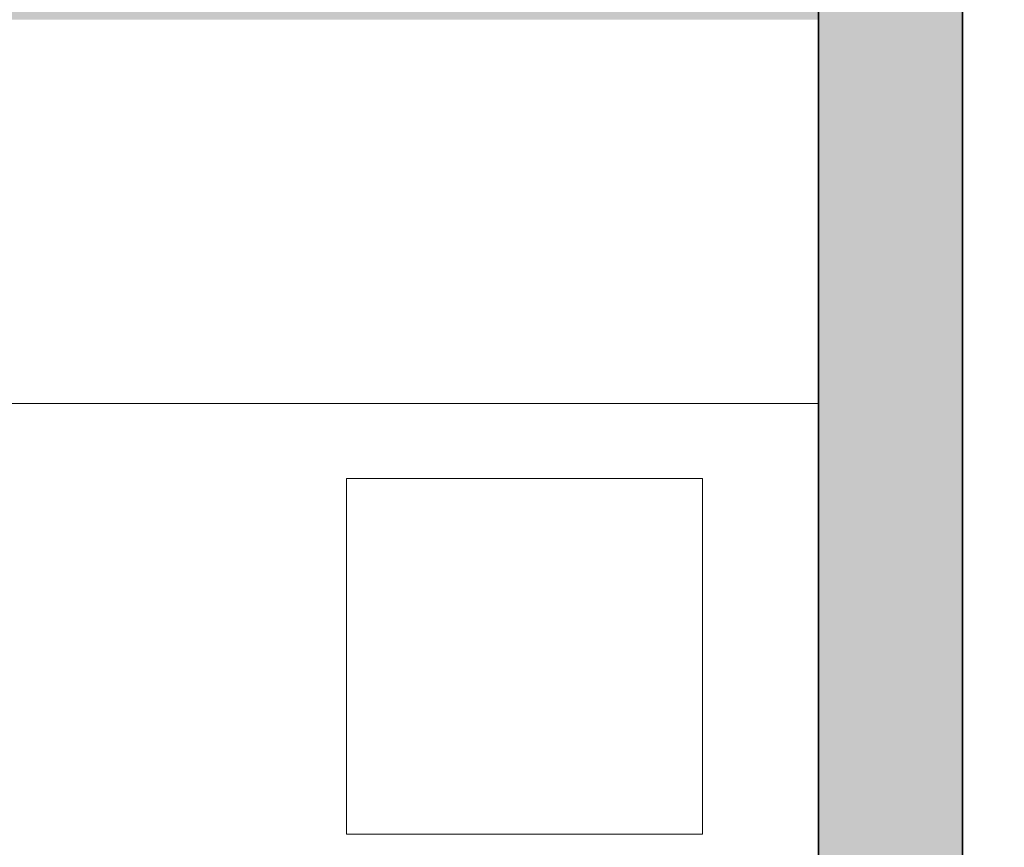
# Model space of a CAD drawing. Units: inches. Extents: x 2083 to 3317, y 1141 to 2115.
# Tile 244 of 256: x 3068 to 3130, y 1365 to 1416. Entities that reach past the tile are written whole.
import ezdxf

# ---------------------------------------------------------------- set-up
doc = ezdxf.new("R2010")
doc.units = ezdxf.units.IN
for name, color, linetype, lineweight in [('A-ANNO-DIMS', 2, 'Continuous', 18), ('A-FLOR-CASE', 8, 'Continuous', 18), ('A-FURN', 8, 'Continuous', 18), ('A-WALL', 7, 'Continuous', 35)]:
    doc.layers.add(name, color=color, linetype=linetype, lineweight=lineweight)
doc.layers.add('A-WALL-PATT', color=251, linetype='Continuous', lineweight=13, true_color=0x636466)
doc.styles.get("Standard").update_dxf_attribs({"font": 'arial.ttf'})
doc.dimstyles.new('ISO-25', dxfattribs={"dimtxt": 12, "dimasz": 12, "dimexe": 1.25, "dimexo": 0.625, "dimtad": 1, "dimlunit": 3, "dimtxsty": 'Standard', "dimcen": 2.5, "dimadec": 0, "dimazin": 0, "dimtfac": 1, "dimtmove": 0, "dimatfit": 3, "dimfxl": 1, "dimarcsym": 0})

# ---------------------------------------------------------------- blocks, each defined once
blk = doc.blocks.new('*D9')
at = {"layer": 'A-ANNO-DIMS', "color": 0, "lineweight": -2, "transparency": 16777216}
for p, q in [((3127.585, 1486.761), (3190.403, 1486.761)), ((3189.153, 1474.761), (3189.153, 1275.261)), ((3127.585, 1263.261), (3190.403, 1263.261))]:
    blk.add_line(p, q, dxfattribs=at)
at = {"layer": 'A-ANNO-DIMS', "color": 0, "transparency": 16777216}
for points in [[(3187.153, 1474.761), (3191.153, 1474.761), (3189.153, 1486.761)], [(3187.153, 1275.261), (3191.153, 1275.261), (3189.153, 1263.261)]]:
    blk.add_solid(points, dxfattribs=at)
at = {"layer": 'Defpoints', "color": 0, "transparency": 16777216}
for p in [(3126.96, 1486.761), (3126.96, 1263.261), (3189.153, 1263.261)]:
    blk.add_point(p, dxfattribs=at)
at = {"layer": 'A-ANNO-DIMS', "color": 0, "transparency": 16777216, "insert": (3182.401, 1375.011), "char_height": 12, "attachment_point": 5, "rotation": 90}
blk.add_mtext('18\'-7.5"', dxfattribs=at)
blk = doc.blocks.new('CASEWORK-96X24')
blk.add_line((0, 96), (0, 0))
blk = doc.blocks.new('NIGHTSTAND-COMPACT')
blk.add_lwpolyline([(22.254, 22.255), (22.254, 0), (0, 0), (0, 22.255)], close=True)
blk = doc.blocks.new('*D35')
at = {"layer": 'A-ANNO-DIMS', "color": 0, "lineweight": -2, "transparency": 16777216}
for p, q in [((3127.585, 2020.761), (3180.56, 2020.761)), ((3179.31, 1275.261), (3179.31, 2008.761)), ((3127.585, 1263.261), (3180.56, 1263.261))]:
    blk.add_line(p, q, dxfattribs=at)
at = {"layer": 'A-ANNO-DIMS', "color": 0, "transparency": 16777216}
for points in [[(3177.31, 2008.761), (3181.31, 2008.761), (3179.31, 2020.761)], [(3177.31, 1275.261), (3181.31, 1275.261), (3179.31, 1263.261)]]:
    blk.add_solid(points, dxfattribs=at)
at = {"layer": 'Defpoints', "color": 0, "transparency": 16777216}
for p in [(3126.96, 2020.761), (3179.31, 2020.761), (3126.96, 1263.261)]:
    blk.add_point(p, dxfattribs=at)
at = {"layer": 'A-ANNO-DIMS', "color": 0, "transparency": 16777216, "insert": (3172.476, 1642.011), "char_height": 12, "attachment_point": 5, "rotation": 90}
blk.add_mtext('63\'-1 1/2"', dxfattribs=at)

msp = doc.modelspace()

# ---------------------------------------------------------------- hatches: boundary and pattern name
at = {"layer": 'A-WALL-PATT'}
h = msp.add_hatch(color=256, dxfattribs=at)
h.dxf.hatch_style = 1
h.paths.add_polyline_path([(3126.96, 2020.761), (2748.96, 2020.761), (2604.96, 2020.761), (2226.96, 2020.761), (2226.96, 1702.761), (2466.96, 1702.761), (2466.96, 1582.761), (2418.96, 1582.761), (2418.96, 1477.761), (2226.96, 1477.761), (2226.96, 1263.261), (2544.96, 1263.261), (2544.96, 1411.761), (2604.96, 1411.761), (2685.96, 1411.761), (2685.96, 1420.761), (2604.96, 1420.761), (2604.96, 1573.761), (2604.96, 1702.761), (2604.96, 2011.761), (2748.96, 2011.761), (2748.96, 1702.761), (2862.96, 1702.761), (2862.96, 1621.761), (2871.96, 1621.761), (2871.96, 1702.761), (2883.96, 1702.761), (2883.96, 1706.939, -0.026459), (2883.96, 1711.761), (2757.96, 1711.761), (2757.96, 1807.761), (2787.96, 1807.761), (2787.96, 1812.261), (2757.96, 1812.261), (2757.96, 2011.761), (2877.96, 2011.761), (2877.96, 1812.261), (2847.96, 1812.261), (2847.96, 1807.761), (2889.836, 1807.761), (2889.836, 1812.261), (2882.46, 1812.261), (2882.46, 2011.761), (3117.96, 2011.761), (3117.96, 1812.261), (2937.836, 1812.261), (2937.836, 1807.761), (2995.71, 1807.761), (2995.71, 1796.118), (3000.21, 1796.118), (3000.21, 1807.761), (3117.96, 1807.761), (3117.96, 1711.761), (3000.21, 1711.761), (3000.21, 1760.118), (2998.573, 1760.118, -0.020711), (2995.71, 1760.118), (2995.71, 1711.761), (2931.96, 1711.761), (2931.96, 1702.761), (3126.96, 1702.761)])
h.paths.add_polyline_path([(2471.46, 2011.761), (2471.46, 1810.011), (2462.717, 1810.011), (2462.717, 1805.511), (2505.96, 1805.511), (2505.96, 1810.011), (2475.96, 1810.011), (2475.96, 2011.761), (2595.96, 2011.761), (2595.96, 1810.011), (2565.96, 1810.011), (2565.96, 1805.511), (2595.96, 1805.511), (2595.96, 1711.761), (2235.96, 1711.761), (2235.96, 1805.511), (2353.71, 1805.511), (2353.71, 1796.054), (2358.21, 1796.054), (2358.21, 1805.511), (2414.717, 1805.511), (2414.717, 1810.011), (2235.96, 1810.011), (2235.96, 2011.761)], flags=16)
h.paths.add_polyline_path([(2270.205, 1994.61), (2270.205, 1970.61), (2246.205, 1970.61), (2246.205, 1994.61)], flags=0)
edge = h.paths.add_edge_path(flags=0)
edge.add_ellipse((2332.027, 1899.798), major_axis=(-3.043, 3.043), ratio=0.168252, start_angle=-161.33217, end_angle=-156.30711, ccw=False)
edge.add_ellipse((2333.082, 1898.744), major_axis=(-1.055, 1.055), ratio=0.453532, start_angle=-123.37102, end_angle=-94.15911)
edge = h.paths.add_edge_path(flags=0)
edge.add_ellipse((2332.027, 1968.876), major_axis=(3.043, 3.043), ratio=0.168252, start_angle=18.66783, end_angle=23.69289)
edge.add_spline(control_points=[(2332.926, 1970.691), (2332.227, 1970.336), (2330.894, 1969.659), (2328.413, 1970.932), (2327.204, 1967.749), (2324.71, 1969.956), (2322.533, 1967.012), (2320.013, 1971.296), (2317.68, 1968.158), (2316.041, 1967.102), (2315.427, 1966.81)], knot_values=[0, 0, 0, 0, 2.267059, 4.324559, 6.685584, 8.878641, 11.121502, 14.300359, 17.755284, 19.732645, 19.732645, 19.732645, 19.732645], degree=3, periodic=0)
edge.add_ellipse((2332.027, 1968.876), major_axis=(3.043, 3.043), ratio=0.168252, start_angle=18.66783, end_angle=23.69289, ccw=False)
edge.add_ellipse((2333.082, 1969.931), major_axis=(1.055, 1.055), ratio=0.453532, start_angle=56.62898, end_angle=85.84089, ccw=False)
edge = h.paths.add_edge_path(flags=0)
edge.add_spline(control_points=[(2296.428, 1967.988), (2293.628, 1965.336), (2287.704, 1959.727), (2299.744, 1949.996), (2294.533, 1935.669), (2290.573, 1920.604), (2293.394, 1909.974), (2296.185, 1904.967)], knot_values=[0.099185, 0.099185, 0.099185, 0.099185, 0.345301, 0.619822, 0.982653, 1.386093, 1.810555, 1.810555, 1.810555, 1.810555], degree=3, periodic=0)
edge.add_spline(control_points=[(2296.185, 1904.967), (2297.384, 1902.619), (2298.001, 1901.949), (2298.553, 1901.468)], knot_values=[0.006246, 0.006246, 0.006246, 0.006246, 0.055476, 0.055476, 0.055476, 0.055476], degree=3, periodic=0)
edge.add_spline(control_points=[(2298.553, 1901.468), (2297.259, 1900.923), (2295.225, 1900.232), (2293.06, 1900.614), (2292.101, 1900.788), (2292.09, 1900.791)], knot_values=[0.312835, 0.312835, 0.312835, 0.312835, 0.40178, 0.474987, 0.475903, 0.475903, 0.475903, 0.475903], degree=3, periodic=0)
edge.add_arc((2292.794, 1904.664), 3.937, 215.4209, 259.69818, ccw=False)
edge.add_spline(control_points=[(2289.585, 1902.382), (2289.477, 1902.535), (2289.368, 1902.688), (2289.261, 1902.841)], knot_values=[0.102872, 0.102872, 0.102872, 0.102872, 0.116896, 0.116896, 0.116896, 0.116896], degree=3, periodic=0)
edge.add_spline(control_points=[(2289.261, 1902.841), (2288.687, 1902.55), (2287.64, 1902.02), (2285.881, 1901.874), (2283.853, 1901.504), (2281.72, 1899.711), (2278.467, 1899.493), (2276.157, 1901.883), (2272.259, 1899.804), (2267.778, 1901.843), (2262.244, 1900.184), (2257.415, 1901.782), (2254.318, 1900.726), (2253.178, 1900.337)], knot_values=[0, 0, 0, 0, 1.907977, 3.477176, 5.261074, 7.972851, 11.680248, 13.717921, 16.939592, 22.789562, 27.502503, 33.595215, 37.145618, 37.145618, 37.145618, 37.145618], degree=3, periodic=0)
edge.add_line((2253.178, 1900.337), (2250.244, 1902.841))
edge.add_line((2250.244, 1902.841), (2250.244, 1965.833))
edge.add_line((2250.244, 1965.833), (2253.178, 1968.337))
edge.add_spline(control_points=[(2253.178, 1968.337), (2254.318, 1967.948), (2257.415, 1966.892), (2262.244, 1968.49), (2267.778, 1966.831), (2271.527, 1968.537), (2273.876, 1967.828), (2274.207, 1967.728)], knot_values=[0, 0, 0, 0, 0.09018, 0.244935, 0.364644, 0.513233, 0.537855, 0.537855, 0.537855, 0.537855], degree=3, periodic=0)
edge.add_arc((2274.353, 1963.793), 3.937, 72.05113, 92.12795, ccw=False)
edge.add_arc((2281.297, 1985.23), 18.596, 252.05113, 288.56572)
edge.add_arc((2292.317, 1956.029), 12.646, 71.02679, 113.77822, ccw=False)
edge = h.paths.add_edge_path(flags=0)
edge.add_spline(control_points=[(2274.899, 1951.856), (2275.066, 1951.617), (2275.233, 1951.377), (2275.398, 1951.136)], knot_values=[1.409916, 1.409916, 1.409916, 1.409916, 1.43159, 1.43159, 1.43159, 1.43159], degree=3, periodic=0)
edge.add_spline(control_points=[(2275.398, 1951.136), (2275.792, 1950.562), (2276.179, 1949.984), (2276.546, 1949.397)], knot_values=[1.358238, 1.358238, 1.358238, 1.358238, 1.409916, 1.409916, 1.409916, 1.409916], degree=3, periodic=0)
edge.add_line((2276.546, 1949.397), (2277.437, 1947.862))
edge.add_spline(control_points=[(2277.437, 1947.862), (2276.304, 1945.673), (2274.64, 1942.427), (2274.632, 1938.094), (2272.799, 1930.852), (2274.356, 1943.897), (2275.948, 1947.923), (2276.546, 1949.397)], knot_values=[0.005632, 0.005632, 0.005632, 0.005632, 0.186014, 0.266002, 0.357087, 0.59639, 0.739732, 0.739732, 0.739732, 0.739732], degree=3, periodic=0)
edge.add_spline(control_points=[(2276.546, 1949.397), (2276.179, 1949.984), (2275.792, 1950.562), (2275.398, 1951.136)], knot_values=[1.358238, 1.358238, 1.358238, 1.358238, 1.409916, 1.409916, 1.409916, 1.409916], degree=3, periodic=0)
edge.add_spline(control_points=[(2275.398, 1951.136), (2274.943, 1950.08), (2274.208, 1948.025), (2273.935, 1944.851), (2272.469, 1937.627), (2273.466, 1945.696), (2274.701, 1951.059), (2274.899, 1951.856)], knot_values=[0.104364, 0.104364, 0.104364, 0.104364, 0.189636, 0.269624, 0.36071, 0.600013, 0.644622, 0.644622, 0.644622, 0.644622], degree=3, periodic=0)
h.paths.add_polyline_path([(2269.168, 1963.128, -0.357527), (2268.171, 1960.976, -0.092561), (2268.171, 1939.436, -0.357527), (2269.168, 1937.285, -0.357527), (2267.016, 1938.282, -0.164785), (2254.686, 1938.282, -0.357527), (2252.534, 1937.285, -0.357527), (2253.531, 1939.436, -0.092561), (2253.531, 1960.976, -0.357527), (2252.534, 1963.128, -0.357527), (2254.686, 1962.131, -0.164785), (2267.016, 1962.131, -0.357527)], flags=0)
h.paths.add_polyline_path([(2248.874, 1967.802), (2248.874, 1957.028), (2249.458, 1957.028), (2249.458, 1911.647), (2248.874, 1911.647), (2248.874, 1900.873), (2246.512, 1900.873, 0.197327), (2244.15, 1902.457), (2244.15, 1966.218, 0.197327), (2246.512, 1967.802)], flags=0)
h.paths.add_polyline_path([(2269.168, 1931.389, -0.357527), (2268.171, 1929.238, -0.092561), (2268.171, 1907.698, -0.357527), (2269.168, 1905.547, -0.357527), (2267.016, 1906.544, -0.164785), (2254.686, 1906.544, -0.357527), (2252.534, 1905.547, -0.357527), (2253.531, 1907.698, -0.092561), (2253.531, 1929.238, -0.357527), (2252.534, 1931.389, -0.357527), (2254.686, 1930.392, -0.164785), (2267.016, 1930.392, -0.357527)], flags=0)
edge = h.paths.add_edge_path(flags=0)
edge.add_spline(control_points=[(2276.197, 1906.724), (2276.168, 1909.029), (2276.114, 1913.372), (2270.598, 1924.925), (2273.905, 1919.013), (2275.922, 1916.262), (2275.475, 1912.402), (2277.258, 1910.381), (2276.696, 1908.225), (2276.646, 1906.813), (2276.618, 1906.008)], knot_values=[0, 0, 0, 0, 8.61026, 16.221274, 18.843057, 23.804898, 27.440828, 29.356102, 31.203478, 33.650687, 33.650687, 33.650687, 33.650687], degree=3, periodic=0)
edge.add_spline(control_points=[(2276.618, 1906.008), (2276.623, 1905.624), (2276.498, 1904.629), (2275.442, 1903.855), (2274.937, 1903.08), (2274.859, 1902.841)], knot_values=[0.156488, 0.156488, 0.156488, 0.156488, 0.184398, 0.231376, 0.250598, 0.250598, 0.250598, 0.250598], degree=3, periodic=0)
edge.add_line((2274.859, 1902.841), (2276.506, 1902.841))
edge.add_spline(control_points=[(2276.506, 1902.841), (2276.788, 1903.085), (2277.665, 1904.125), (2278.25, 1904.341), (2277.654, 1908.527), (2278.156, 1906.228), (2278.1, 1905.286), (2278.847, 1904.069), (2277.857, 1903.415), (2277.874, 1902.991), (2277.904, 1902.841)], knot_values=[0.059574, 0.059574, 0.059574, 0.059574, 0.080753, 0.103741, 0.16972, 0.176036, 0.207137, 0.240474, 0.262341, 0.27366, 0.27366, 0.27366, 0.27366], degree=3, periodic=0)
edge.add_line((2277.904, 1902.841), (2280.03, 1902.841))
edge.add_spline(control_points=[(2280.03, 1902.841), (2279.888, 1903.088), (2279.499, 1903.982), (2280.152, 1905.939), (2278.104, 1909.658), (2279.762, 1907.185), (2280.328, 1904.875), (2280.485, 1903.49), (2281.463, 1903.249), (2281.758, 1902.936), (2281.834, 1902.841)], knot_values=[0.013856, 0.013856, 0.013856, 0.013856, 0.034874, 0.088867, 0.107879, 0.126738, 0.158714, 0.193757, 0.217487, 0.226722, 0.226722, 0.226722, 0.226722], degree=3, periodic=0)
edge.add_spline(control_points=[(2281.834, 1902.841), (2281.788, 1902.827), (2281.647, 1902.783), (2281.396, 1902.859), (2281.088, 1902.985), (2280.721, 1903.061), (2280.333, 1903.026), (2280.125, 1902.899), (2280.03, 1902.841)], knot_values=[0, 0, 0, 0, 0.14413, 0.435517, 0.749276, 1.153046, 1.548371, 1.878348, 1.878348, 1.878348, 1.878348], degree=3, periodic=0)
edge.add_line((2280.03, 1902.841), (2277.904, 1902.841))
edge.add_spline(control_points=[(2277.904, 1902.841), (2277.893, 1902.796), (2277.865, 1902.68), (2277.607, 1902.687), (2277.274, 1902.801), (2276.838, 1902.62), (2276.584, 1902.789), (2276.506, 1902.841)], knot_values=[0, 0, 0, 0, 0.127189, 0.326199, 0.628009, 1.24357, 1.515331, 1.515331, 1.515331, 1.515331], degree=3, periodic=0)
edge.add_line((2276.506, 1902.841), (2274.859, 1902.841))
edge.add_spline(control_points=[(2274.859, 1902.841), (2274.814, 1902.899), (2274.725, 1903.013), (2274.493, 1903.119), (2274.244, 1902.961), (2273.937, 1903.185), (2273.614, 1902.983), (2273.408, 1902.883), (2273.322, 1902.841)], knot_values=[0, 0, 0, 0, 0.21843, 0.436957, 0.687977, 0.990379, 1.398396, 1.69185, 1.69185, 1.69185, 1.69185], degree=3, periodic=0)
edge.add_spline(control_points=[(2273.322, 1902.841), (2273.617, 1903.446), (2274.274, 1904.538), (2276.027, 1904.574), (2276.207, 1906.584), (2276.197, 1906.724)], knot_values=[0.012227, 0.012227, 0.012227, 0.012227, 0.059472, 0.106218, 0.134458, 0.134458, 0.134458, 0.134458], degree=3, periodic=0)
h.paths.add_polyline_path([(2270.776, 1897.79), (2270.776, 1873.79), (2246.776, 1873.79), (2246.776, 1897.79)], flags=0)
h.paths.add_polyline_path([(2353.71, 1760.005), (2353.71, 1760.054), (2358.21, 1760.054, -0.033729)], flags=0)
h.paths.add_polyline_path([(2321.819, 1737.529), (2341.995, 1737.529, -0.414214), (2343.203, 1736.321), (2343.203, 1721.021, -0.414214), (2341.995, 1719.813), (2321.819, 1719.813, -0.414214), (2320.611, 1721.021), (2320.611, 1736.321, -0.414214)], flags=0)
h.paths.add_polyline_path([(2324.235, 1736.321), (2339.579, 1736.321, -0.414214), (2341.995, 1733.905), (2341.995, 1725.45, -0.414214), (2339.579, 1723.034), (2333.681, 1723.034), (2333.845, 1722.045, -0.870646), (2335.425, 1721.826, -0.767327), (2333.923, 1721.423), (2331.291, 1721.423, -0.767327), (2329.788, 1721.826, -0.870646), (2331.368, 1722.045), (2331.533, 1723.034), (2324.235, 1723.034, -0.414214), (2321.819, 1725.45), (2321.819, 1733.905, -0.414214)], flags=0)
h.paths.add_polyline_path([(2570.484, 1928.615), (2589.684, 1928.615), (2590.169, 1928.615), (2590.169, 1904.993), (2570.484, 1904.993)], flags=0)
h.paths.add_polyline_path([(2574.447, 1927.264, -1), (2572.829, 1927.264, -1)], flags=0)
h.paths.add_polyline_path([(2573.09, 1926.941), (2573.925, 1927.776), (2574.148, 1927.553), (2573.313, 1926.718)], flags=0)
h.paths.add_polyline_path([(2578.779, 1919.73, -1), (2571.592, 1919.73, -1)], flags=0)
h.paths.add_polyline_path([(2578.385, 1919.73, -1), (2571.985, 1919.73, -1)], flags=0)
h.paths.add_polyline_path([(2331.596, 1729.476, -1), (2333.618, 1729.476, -1)], flags=0)
h.paths.add_polyline_path([(2578.034, 1927.264, -1), (2576.416, 1927.264, -1)], flags=0)
h.paths.add_polyline_path([(2576.689, 1927.531), (2576.912, 1927.754), (2577.747, 1926.919), (2577.524, 1926.696)], flags=0)
h.paths.add_polyline_path([(2578.139, 1909.86, -1), (2572.232, 1909.86, -1)], flags=0)
h.paths.add_polyline_path([(2577.745, 1909.86, -1), (2572.625, 1909.86, -1)], flags=0)
h.paths.add_polyline_path([(2583.798, 1927.264, -1), (2582.179, 1927.264, -1)], flags=0)
h.paths.add_polyline_path([(2582.719, 1927.754), (2583.554, 1926.919), (2583.331, 1926.696), (2582.496, 1927.531)], flags=0)
h.paths.add_polyline_path([(2582.496, 1927.531), (2582.719, 1927.754), (2583.554, 1926.919), (2583.331, 1926.696)], flags=0)
h.paths.add_polyline_path([(2587.739, 1920.53, -1), (2581.832, 1920.53, -1)], flags=0)
h.paths.add_polyline_path([(2587.345, 1920.53, -1), (2582.225, 1920.53, -1)], flags=0)
h.paths.add_polyline_path([(2587.385, 1927.264, -1), (2585.766, 1927.264, -1)], flags=0)
h.paths.add_polyline_path([(2586.082, 1926.98), (2586.917, 1927.815), (2587.14, 1927.593), (2586.305, 1926.758)], flags=0)
h.paths.add_polyline_path([(2588.379, 1910.66, -1), (2581.192, 1910.66, -1)], flags=0)
h.paths.add_polyline_path([(2587.985, 1910.66, -1), (2581.585, 1910.66, -1)], flags=0)
h.paths.add_polyline_path([(2417.168, 1729.478), (2437.344, 1729.478, -0.414214), (2438.552, 1728.27), (2438.552, 1712.969, -0.414214), (2437.344, 1711.761), (2417.168, 1711.761, -0.414214), (2415.96, 1712.969), (2415.96, 1728.27, -0.414214)], flags=0)
h.paths.add_polyline_path([(2419.584, 1728.27), (2434.928, 1728.27, -0.414214), (2437.344, 1725.854), (2437.344, 1717.398, -0.414214), (2434.928, 1714.983), (2429.029, 1714.983), (2429.194, 1713.994, -0.870646), (2430.774, 1713.775, -0.767327), (2429.271, 1713.372), (2426.64, 1713.372, -0.767327), (2425.137, 1713.775, -0.870646), (2426.717, 1713.994), (2426.882, 1714.983), (2419.584, 1714.983, -0.414214), (2417.168, 1717.398), (2417.168, 1725.854, -0.414214)], flags=0)
h.paths.add_polyline_path([(2419.584, 1728.27), (2434.928, 1728.27, -0.414214), (2437.344, 1725.854), (2437.344, 1717.398, -0.414214), (2434.928, 1714.983), (2429.029, 1714.983), (2428.358, 1719.009), (2427.553, 1719.009), (2426.882, 1714.983), (2419.584, 1714.983, -0.414214), (2417.168, 1717.398), (2417.168, 1725.854, -0.414214)], flags=0)
h.paths.add_polyline_path([(2426.944, 1721.425, -1), (2428.967, 1721.425, -1)], flags=0)
h.paths.add_polyline_path([(2475.96, 1702.761), (2595.96, 1702.761), (2595.96, 1582.761), (2475.96, 1582.761)], flags=16)
h.paths.add_polyline_path([(2427.96, 1573.761), (2595.96, 1573.761), (2595.96, 1468.761), (2595.96, 1420.761), (2384.46, 1420.761), (2384.46, 1468.761), (2427.96, 1468.761)], flags=16)
h.paths.add_polyline_path([(2379.96, 1468.761), (2379.96, 1420.761), (2235.96, 1420.761), (2235.96, 1468.761)], flags=16)
h.paths.add_polyline_path([(2317.816, 1466.696), (2337.992, 1466.696, -0.414214), (2339.2, 1465.488), (2339.2, 1450.187, -0.414214), (2337.992, 1448.979), (2317.816, 1448.979, -0.414214), (2316.608, 1450.187), (2316.608, 1465.488, -0.414214)], flags=0)
h.paths.add_polyline_path([(2320.232, 1465.488), (2335.576, 1465.488, -0.414214), (2337.992, 1463.072), (2337.992, 1454.616, -0.414214), (2335.576, 1452.2), (2329.677, 1452.2), (2329.842, 1451.212, -0.870646), (2331.422, 1450.992, -0.767327), (2329.92, 1450.59), (2327.288, 1450.59, -0.767327), (2325.785, 1450.992, -0.870646), (2327.365, 1451.212), (2327.53, 1452.2), (2320.232, 1452.2, -0.414214), (2317.816, 1454.616), (2317.816, 1463.072, -0.414214)], flags=0)
h.paths.add_polyline_path([(2320.232, 1465.488), (2335.576, 1465.488, -0.414214), (2337.992, 1463.072), (2337.992, 1454.616, -0.414214), (2335.576, 1452.2), (2329.677, 1452.2), (2329.006, 1456.227), (2328.201, 1456.227), (2327.53, 1452.2), (2320.232, 1452.2, -0.414214), (2317.816, 1454.616), (2317.816, 1463.072, -0.414214)], flags=0)
h.paths.add_polyline_path([(2327.593, 1458.643, -1), (2329.615, 1458.643, -1)], flags=0)
h.paths.add_polyline_path([(2244.412, 1433.34), (2241.921, 1433.34, -0.414214), (2240.018, 1435.244), (2240.018, 1440.953, -0.414211), (2241.921, 1442.856), (2244.412, 1442.856, -1.976472)], flags=0)
h.paths.add_polyline_path([(2245.357, 1434.398, -0.414214), (2245.357, 1441.799, -2.144098)], flags=0)
h.paths.add_polyline_path([(2535.96, 1416.261), (2535.96, 1272.261), (2235.96, 1272.261), (2235.96, 1416.261)], flags=16)
h.paths.add_polyline_path([(2260.12, 1384.293), (2260.12, 1362.039), (2237.865, 1362.039), (2237.865, 1384.293)], flags=0)
edge = h.paths.add_edge_path(flags=0)
edge.add_line((2318.252, 1362.093), (2318.146, 1362.001))
edge.add_ellipse((2317.445, 1360.431), major_axis=(2.822, 2.822), ratio=0.168252, start_angle=18.66783, end_angle=20.94813, ccw=False)
edge.add_ellipse((2318.423, 1361.409), major_axis=(0.978, 0.978), ratio=0.453532, start_angle=56.62898, end_angle=70.2262, ccw=False)
edge = h.paths.add_edge_path(flags=0)
edge.add_line((2319.107, 1295.571), (2319.015, 1295.677))
edge.add_ellipse((2317.445, 1296.378), major_axis=(-2.822, 2.822), ratio=0.168252, start_angle=-161.33217, end_angle=-159.05187, ccw=False)
edge.add_ellipse((2318.423, 1295.4), major_axis=(-0.978, 0.978), ratio=0.453532, start_angle=-123.37102, end_angle=-109.7738)
edge = h.paths.add_edge_path(flags=0)
edge.add_spline(control_points=[(2284.21, 1301.17), (2284.581, 1300.445), (2284.891, 1299.892), (2285.16, 1299.461)], knot_values=[0.039066, 0.039066, 0.039066, 0.039066, 0.055476, 0.055476, 0.055476, 0.055476], degree=3, periodic=0)
edge.add_line((2285.16, 1299.461), (2284.21, 1301.17))
edge = h.paths.add_edge_path(flags=0)
edge.add_line((2280.412, 1297.298), (2283.37, 1297.036))
edge.add_line((2283.37, 1297.036), (2286.406, 1297.926))
edge.add_spline(control_points=[(2286.406, 1297.926), (2285.305, 1297.463), (2284.345, 1297.129), (2283.37, 1297.036)], knot_values=[0.394369, 0.394369, 0.394369, 0.394369, 0.475903, 0.475903, 0.475903, 0.475903], degree=3, periodic=0)
edge.add_spline(control_points=[(2283.37, 1297.036), (2283.281, 1297.028), (2282.316, 1296.957), (2281.313, 1297.134), (2280.423, 1297.296), (2280.412, 1297.298)], knot_values=[0.312835, 0.312835, 0.312835, 0.312835, 0.320246, 0.393453, 0.394369, 0.394369, 0.394369, 0.394369], degree=3, periodic=0)
edge = h.paths.add_edge_path(flags=0)
edge.add_line((2284.436, 1359.607), (2280.446, 1355.328))
edge.add_line((2280.446, 1355.328), (2279.58, 1351.018))
edge.add_line((2279.58, 1351.018), (2282.413, 1346.58))
edge.add_spline(control_points=[(2282.413, 1346.58), (2283.153, 1345.589), (2284.253, 1344.029), (2284.801, 1342.387), (2284.935, 1341.806)], knot_values=[1.240098, 1.240098, 1.240098, 1.240098, 1.332892, 1.382712, 1.382712, 1.382712, 1.382712], degree=3, periodic=0)
edge.add_spline(control_points=[(2284.935, 1341.806), (2285.319, 1340.141), (2285.233, 1338.409), (2284.91, 1336.654)], knot_values=[1.097484, 1.097484, 1.097484, 1.097484, 1.240098, 1.240098, 1.240098, 1.240098], degree=3, periodic=0)
edge.add_spline(control_points=[(2284.91, 1336.654), (2284.587, 1334.899), (2284.027, 1333.12), (2283.463, 1331.361)], knot_values=[0.95487, 0.95487, 0.95487, 0.95487, 1.097484, 1.097484, 1.097484, 1.097484], degree=3, periodic=0)
edge.add_line((2283.463, 1331.361), (2281.89, 1326.153))
edge.add_line((2281.89, 1326.153), (2280.756, 1321.056))
edge.add_line((2280.756, 1321.056), (2280.299, 1316.002))
edge.add_line((2280.299, 1316.002), (2280.716, 1310.95))
edge.add_line((2280.716, 1310.95), (2282.028, 1305.972))
edge.add_line((2282.028, 1305.972), (2284.21, 1301.17))
edge.add_spline(control_points=[(2284.21, 1301.17), (2283.341, 1302.73), (2282.612, 1304.336), (2282.028, 1305.972)], knot_values=[0.099185, 0.099185, 0.099185, 0.099185, 0.241799, 0.241799, 0.241799, 0.241799], degree=3, periodic=0)
edge.add_spline(control_points=[(2282.028, 1305.972), (2281.444, 1307.608), (2281.005, 1309.273), (2280.716, 1310.95)], knot_values=[0.241799, 0.241799, 0.241799, 0.241799, 0.384413, 0.384413, 0.384413, 0.384413], degree=3, periodic=0)
edge.add_spline(control_points=[(2280.716, 1310.95), (2280.433, 1312.588), (2280.289, 1314.277), (2280.299, 1315.962), (2280.299, 1316.002)], knot_values=[0.384413, 0.384413, 0.384413, 0.384413, 0.523647, 0.527028, 0.527028, 0.527028, 0.527028], degree=3, periodic=0)
edge.add_spline(control_points=[(2280.299, 1316.002), (2280.312, 1317.687), (2280.478, 1319.368), (2280.756, 1321.056)], knot_values=[0.527028, 0.527028, 0.527028, 0.527028, 0.669642, 0.669642, 0.669642, 0.669642], degree=3, periodic=0)
edge.add_spline(control_points=[(2280.756, 1321.056), (2281.035, 1322.744), (2281.426, 1324.44), (2281.89, 1326.153)], knot_values=[0.669642, 0.669642, 0.669642, 0.669642, 0.812256, 0.812256, 0.812256, 0.812256], degree=3, periodic=0)
edge.add_spline(control_points=[(2281.89, 1326.153), (2282.264, 1327.533), (2282.788, 1329.262), (2283.353, 1331.018), (2283.463, 1331.361)], knot_values=[0.812256, 0.812256, 0.812256, 0.812256, 0.927087, 0.95487, 0.95487, 0.95487, 0.95487], degree=3, periodic=0)
edge.add_line((2283.463, 1331.361), (2284.91, 1336.654))
edge.add_line((2284.91, 1336.654), (2284.935, 1341.806))
edge.add_line((2284.935, 1341.806), (2282.413, 1346.58))
edge.add_spline(control_points=[(2282.413, 1346.58), (2281.275, 1348.104), (2280.078, 1349.57), (2279.58, 1351.018)], knot_values=[1.382712, 1.382712, 1.382712, 1.382712, 1.525326, 1.525326, 1.525326, 1.525326], degree=3, periodic=0)
edge.add_spline(control_points=[(2279.58, 1351.018), (2279.443, 1351.415), (2279.136, 1352.857), (2279.735, 1354.29), (2280.446, 1355.328)], knot_values=[1.525326, 1.525326, 1.525326, 1.525326, 1.564439, 1.667941, 1.667941, 1.667941, 1.667941], degree=3, periodic=0)
edge.add_spline(control_points=[(2280.446, 1355.328), (2281.426, 1356.758), (2282.931, 1358.183), (2284.436, 1359.607)], knot_values=[1.667941, 1.667941, 1.667941, 1.667941, 1.810555, 1.810555, 1.810555, 1.810555], degree=3, periodic=0)
edge.add_arc((2280.623, 1348.518), 11.726, 71.02679, 113.77822)
edge.add_arc((2270.405, 1375.595), 17.244, 252.05113, 288.56572, ccw=False)
edge.add_arc((2263.966, 1355.718), 3.651, 72.05113, 92.12795)
edge.add_arc((2263.966, 1355.718), 3.651, 92.12795, 177.98513)
edge.add_spline(control_points=[(2260.318, 1355.846), (2260.26, 1354.221), (2260.551, 1350.187), (2262.999, 1346.766), (2264.473, 1344.649)], knot_values=[1.43159, 1.43159, 1.43159, 1.43159, 1.564144, 1.770695, 1.770695, 1.770695, 1.770695], degree=3, periodic=0)
edge.add_line((2264.473, 1344.649), (2264.936, 1343.983))
edge.add_spline(control_points=[(2263.801, 1340.248), (2263.843, 1340.514), (2264.067, 1341.756), (2264.513, 1343.002), (2264.935, 1343.981)], knot_values=[0.53657, 0.53657, 0.53657, 0.53657, 0.559349, 0.644622, 0.644622, 0.644622, 0.644622], degree=3, periodic=0)
edge.add_spline(control_points=[(2264.935, 1343.981), (2265.118, 1343.715), (2265.299, 1343.448), (2265.477, 1343.179)], knot_values=[1.384077, 1.384077, 1.384077, 1.384077, 1.409916, 1.409916, 1.409916, 1.409916], degree=3, periodic=0)
edge.add_spline(control_points=[(2265.477, 1343.179), (2265.655, 1342.911), (2265.829, 1342.641), (2265.999, 1342.369)], knot_values=[1.358238, 1.358238, 1.358238, 1.358238, 1.384077, 1.384077, 1.384077, 1.384077], degree=3, periodic=0)
edge.add_line((2265.999, 1342.369), (2266.826, 1340.946))
edge.add_spline(control_points=[(2266.826, 1340.946), (2268.894, 1337.09), (2271.398, 1325.843), (2270.516, 1310.569), (2275.919, 1301.861), (2277.79, 1299.199)], knot_values=[0.116896, 0.116896, 0.116896, 0.116896, 0.472987, 1.050969, 1.313793, 1.313793, 1.313793, 1.313793], degree=3, periodic=0)
edge.add_spline(control_points=[(2277.79, 1299.199), (2277.839, 1299.128), (2277.889, 1299.057), (2277.94, 1298.987)], knot_values=[0.109884, 0.109884, 0.109884, 0.109884, 0.116896, 0.116896, 0.116896, 0.116896], degree=3, periodic=0)
edge.add_line((2277.94, 1298.987), (2277.789, 1299.199))
edge.add_spline(control_points=[(2277.789, 1299.199), (2277.257, 1298.929), (2276.286, 1298.438), (2275.039, 1298.334), (2274.383, 1298.239), (2274.215, 1298.209)], knot_values=[33.12187, 33.12187, 33.12187, 33.12187, 35.029056, 36.598255, 37.144827, 37.144827, 37.144827, 37.144827], degree=3, periodic=0)
edge.add_line((2274.215, 1298.209), (2273.073, 1297.893))
edge.add_spline(control_points=[(2273.073, 1297.893), (2272.323, 1297.58), (2271.039, 1296.511), (2269.248, 1296.226), (2268.423, 1296.375)], knot_values=[26.532584, 26.532584, 26.532584, 26.532584, 29.198919, 31.839101, 31.839101, 31.839101, 31.839101], degree=3, periodic=0)
edge.add_line((2268.423, 1296.375), (2263.879, 1297.458))
edge.add_spline(control_points=[(2263.879, 1297.458), (2263.556, 1297.359), (2261.86, 1296.839), (2260.239, 1297.282), (2258.933, 1297.516)], knot_values=[15.919551, 15.919551, 15.919551, 15.919551, 16.939592, 21.226067, 21.226067, 21.226067, 21.226067], degree=3, periodic=0)
edge.add_line((2258.933, 1297.516), (2254.055, 1297.329))
edge.add_spline(control_points=[(2254.055, 1297.329), (2253.756, 1297.296), (2252.114, 1297.165), (2250.462, 1297.544), (2249.13, 1297.668)], knot_values=[5.306517, 5.306517, 5.306517, 5.306517, 6.276435, 10.613034, 10.613034, 10.613034, 10.613034], degree=3, periodic=0)
edge.add_line((2249.13, 1297.668), (2244.332, 1296.878))
edge.add_line((2244.332, 1296.878), (2241.611, 1299.199))
edge.add_line((2241.611, 1299.199), (2241.611, 1357.609))
edge.add_line((2241.611, 1357.609), (2244.332, 1359.931))
edge.add_line((2244.332, 1359.931), (2252.729, 1359.543))
edge.add_spline(control_points=[(2252.729, 1359.543), (2252.871, 1359.546), (2253.306, 1359.548), (2253.74, 1359.514), (2254.032, 1359.482)], knot_values=[0.233291, 0.233291, 0.233291, 0.233291, 0.244935, 0.268927, 0.268927, 0.268927, 0.268927], degree=3, periodic=0)
edge.add_line((2254.032, 1359.482), (2259.587, 1359.416))
edge.add_spline(control_points=[(2259.587, 1359.416), (2260.677, 1359.629), (2262.073, 1359.897), (2263.524, 1359.459), (2263.83, 1359.366)], knot_values=[0.422516, 0.422516, 0.422516, 0.422516, 0.513233, 0.537855, 0.537855, 0.537855, 0.537855], degree=3, periodic=0)
edge.add_arc((2263.966, 1355.718), 3.651, 72.05113, 92.12795, ccw=False)
edge.add_arc((2270.405, 1375.595), 17.244, 252.05113, 288.56572)
edge.add_arc((2280.623, 1348.518), 11.726, 71.02679, 113.77822, ccw=False)
h.paths.add_polyline_path([(2240.341, 1359.435), (2240.341, 1349.444), (2240.882, 1349.444), (2240.882, 1307.365), (2240.341, 1307.365), (2240.341, 1297.374), (2238.15, 1297.374, 0.197327), (2235.96, 1298.843), (2235.96, 1357.966, 0.197327), (2238.15, 1359.435)], flags=0)
h.paths.add_polyline_path([(2259.158, 1355.101, -0.357527), (2258.233, 1353.106, -0.092561), (2258.233, 1333.133, -0.357527), (2259.158, 1331.138, -0.357527), (2257.163, 1332.062, -0.164785), (2245.729, 1332.062, -0.357527), (2243.735, 1331.138, -0.357527), (2244.659, 1333.133, -0.092561), (2244.659, 1353.106, -0.357527), (2243.735, 1355.101, -0.357527), (2245.729, 1354.176, -0.164785), (2257.163, 1354.176, -0.357527)], flags=0)
edge = h.paths.add_edge_path(flags=0)
edge.add_line((2265.999, 1342.369), (2266.826, 1340.946))
edge.add_line((2266.826, 1340.946), (2265.308, 1337.814))
edge.add_line((2265.308, 1337.814), (2264.358, 1334.653))
edge.add_line((2264.358, 1334.653), (2264.262, 1333.8))
edge.add_spline(control_points=[(2264.262, 1333.8), (2264.208, 1333.187), (2264.162, 1332.366), (2264.007, 1331.414), (2263.969, 1331.202)], knot_values=[0.464444, 0.464444, 0.464444, 0.464444, 0.516691, 0.531608, 0.531608, 0.531608, 0.531608], degree=3, periodic=0)
edge.add_spline(control_points=[(2263.969, 1331.202), (2263.775, 1330.119), (2263.424, 1328.791), (2263.257, 1328.531), (2263.234, 1328.515)], knot_values=[0.372682, 0.372682, 0.372682, 0.372682, 0.44885, 0.464444, 0.464444, 0.464444, 0.464444], degree=3, periodic=0)
edge.add_spline(control_points=[(2263.234, 1328.515), (2263.096, 1328.42), (2263.131, 1329.301), (2263.275, 1330.616)], knot_values=[0.280919, 0.280919, 0.280919, 0.280919, 0.372682, 0.372682, 0.372682, 0.372682], degree=3, periodic=0)
edge.add_spline(control_points=[(2263.275, 1330.616), (2263.419, 1331.93), (2263.672, 1333.677), (2263.97, 1335.315)], knot_values=[0.189157, 0.189157, 0.189157, 0.189157, 0.280919, 0.280919, 0.280919, 0.280919], degree=3, periodic=0)
edge.add_spline(control_points=[(2263.97, 1335.315), (2264.1, 1336.032), (2264.419, 1337.622), (2264.755, 1338.864), (2264.947, 1339.491)], knot_values=[0.097394, 0.097394, 0.097394, 0.097394, 0.137578, 0.189157, 0.189157, 0.189157, 0.189157], degree=3, periodic=0)
edge.add_spline(control_points=[(2264.947, 1339.491), (2265.29, 1340.606), (2265.644, 1341.494), (2265.999, 1342.369)], knot_values=[0.005632, 0.005632, 0.005632, 0.005632, 0.097394, 0.097394, 0.097394, 0.097394], degree=3, periodic=0)
h.paths.add_polyline_path([(2259.158, 1325.671, -0.357527), (2258.233, 1323.676, -0.092561), (2258.233, 1303.703, -0.357527), (2259.158, 1301.708, -0.357527), (2257.163, 1302.633, -0.164785), (2245.729, 1302.633, -0.357527), (2243.735, 1301.708, -0.357527), (2244.659, 1303.703, -0.092561), (2244.659, 1323.676, -0.357527), (2243.735, 1325.671, -0.357527), (2245.729, 1324.747, -0.164785), (2257.163, 1324.747, -0.357527)], flags=0)
edge = h.paths.add_edge_path(flags=0)
edge.add_spline(control_points=[(2261.709, 1317.311), (2261.679, 1317.418), (2261.762, 1317.389), (2262.491, 1316.09), (2262.962, 1315.301)], knot_values=[14.955861, 14.955861, 14.955861, 14.955861, 16.221274, 18.694826, 18.694826, 18.694826, 18.694826], degree=3, periodic=0)
edge.add_spline(control_points=[(2262.962, 1315.301), (2262.99, 1315.254), (2263.702, 1314.067), (2264.349, 1313.127), (2264.73, 1312.164)], knot_values=[18.694826, 18.694826, 18.694826, 18.694826, 18.843057, 22.433791, 22.433791, 22.433791, 22.433791], degree=3, periodic=0)
edge.add_spline(control_points=[(2264.73, 1312.164), (2264.876, 1311.796), (2265.177, 1310.77), (2265.143, 1309.559), (2265.248, 1308.824)], knot_values=[22.433791, 22.433791, 22.433791, 22.433791, 23.804898, 26.172756, 26.172756, 26.172756, 26.172756], degree=3, periodic=0)
edge.add_line((2265.248, 1308.824), (2265.851, 1307.172))
edge.add_spline(control_points=[(2265.851, 1307.172), (2266.065, 1306.822), (2266.384, 1306.332), (2266.424, 1305.781), (2266.42, 1305.611)], knot_values=[28.062562, 28.062562, 28.062562, 28.062562, 29.356102, 29.911721, 29.911721, 29.911721, 29.911721], degree=3, periodic=0)
edge.add_spline(control_points=[(2266.42, 1305.611), (2266.416, 1305.433), (2266.394, 1305.25), (2266.365, 1305.066)], knot_values=[29.911721, 29.911721, 29.911721, 29.911721, 30.497837, 30.497837, 30.497837, 30.497837], degree=3, periodic=0)
edge.add_line((2266.365, 1305.066), (2266.066, 1302.136))
edge.add_spline(control_points=[(2266.066, 1302.136), (2266.071, 1301.78), (2265.998, 1301.2), (2265.663, 1300.759), (2265.509, 1300.586)], knot_values=[0.156488, 0.156488, 0.156488, 0.156488, 0.184398, 0.203543, 0.203543, 0.203543, 0.203543], degree=3, periodic=0)
edge.add_line((2265.509, 1300.586), (2264.435, 1299.199))
edge.add_line((2264.435, 1299.199), (2265.962, 1299.199))
edge.add_line((2265.962, 1299.199), (2267.336, 1301.175))
edge.add_line((2267.336, 1301.175), (2267.312, 1301.986))
edge.add_spline(control_points=[(2267.312, 1301.986), (2267.261, 1302.862), (2267.16, 1303.737), (2267.271, 1303.326)], knot_values=[0.126229, 0.126229, 0.126229, 0.126229, 0.166617, 0.166617, 0.166617, 0.166617], degree=3, periodic=0)
edge.add_spline(control_points=[(2267.271, 1303.326), (2267.28, 1303.294), (2267.31, 1303.175), (2267.373, 1302.884), (2267.406, 1302.683), (2267.418, 1302.601)], knot_values=[0.166617, 0.166617, 0.166617, 0.166617, 0.16972, 0.176036, 0.180765, 0.180765, 0.180765, 0.180765], degree=3, periodic=0)
edge.add_spline(control_points=[(2267.744, 1300.988), (2267.688, 1301.151), (2267.481, 1301.657), (2267.484, 1302.145), (2267.418, 1302.601)], knot_values=[0.180765, 0.180765, 0.180765, 0.180765, 0.193767, 0.220139, 0.220139, 0.220139, 0.220139], degree=3, periodic=0)
edge.add_line((2267.418, 1302.601), (2267.744, 1300.988))
edge.add_spline(control_points=[(2267.744, 1300.988), (2267.832, 1300.732), (2267.932, 1300.31), (2267.555, 1299.975), (2267.429, 1299.829)], knot_values=[0.220139, 0.220139, 0.220139, 0.220139, 0.240474, 0.25489, 0.25489, 0.25489, 0.25489], degree=3, periodic=0)
edge.add_line((2267.429, 1299.829), (2267.258, 1299.199))
edge.add_line((2267.258, 1299.199), (2269.23, 1299.199))
edge.add_spline(control_points=[(2269.23, 1299.199), (2269.099, 1299.429), (2268.843, 1300.016), (2269.012, 1300.916), (2268.947, 1301.661)], knot_values=[0.013856, 0.013856, 0.013856, 0.013856, 0.034874, 0.067073, 0.067073, 0.067073, 0.067073], degree=3, periodic=0)
edge.add_line((2268.947, 1301.661), (2268.432, 1303.603))
edge.add_spline(control_points=[(2268.432, 1303.603), (2268.176, 1304.192), (2267.596, 1305.251), (2268.041, 1304.623), (2268.251, 1304.282)], knot_values=[0.090155, 0.090155, 0.090155, 0.090155, 0.107879, 0.120289, 0.120289, 0.120289, 0.120289], degree=3, periodic=0)
edge.add_spline(control_points=[(2268.251, 1304.282), (2268.361, 1304.105), (2269.058, 1302.918), (2269.383, 1301.59), (2269.521, 1300.776), (2269.575, 1300.556)], knot_values=[0.120289, 0.120289, 0.120289, 0.120289, 0.126738, 0.158714, 0.173506, 0.173506, 0.173506, 0.173506], degree=3, periodic=0)
edge.add_line((2269.575, 1300.556), (2270.686, 1299.421))
edge.add_spline(control_points=[(2270.686, 1299.421), (2270.767, 1299.357), (2270.838, 1299.281), (2270.903, 1299.199)], knot_values=[0.21816, 0.21816, 0.21816, 0.21816, 0.226722, 0.226722, 0.226722, 0.226722], degree=3, periodic=0)
edge.add_line((2270.937, 1299.193), (2270.903, 1299.199))
edge.add_spline(control_points=[(2270.903, 1299.199), (2270.86, 1299.186), (2270.73, 1299.146), (2270.496, 1299.216), (2270.272, 1299.308), (2270.121, 1299.348), (2270.063, 1299.36)], knot_values=[0.939174, 0.939174, 0.939174, 0.939174, 1.083304, 1.374691, 1.68845, 1.878348, 1.878348, 1.878348, 1.878348], degree=3, periodic=0)
edge.add_line((2270.063, 1299.36), (2269.23, 1299.199))
edge.add_line((2269.23, 1299.199), (2267.258, 1299.199))
edge.add_spline(control_points=[(2267.258, 1299.199), (2267.248, 1299.157), (2267.223, 1299.05), (2266.984, 1299.057), (2266.809, 1299.116), (2266.677, 1299.109), (2266.637, 1299.105)], knot_values=[0.757665, 0.757665, 0.757665, 0.757665, 0.884854, 1.083864, 1.385675, 1.515331, 1.515331, 1.515331, 1.515331], degree=3, periodic=0)
edge.add_spline(control_points=[(2266.637, 1299.105), (2266.485, 1299.089), (2266.236, 1299.017), (2266.035, 1299.151), (2265.962, 1299.199)], knot_values=[0, 0, 0, 0, 0.485905, 0.757665, 0.757665, 0.757665, 0.757665], degree=3, periodic=0)
edge.add_line((2265.962, 1299.199), (2264.435, 1299.199))
edge.add_line((2264.435, 1299.199), (2263.858, 1299.367))
edge.add_spline(control_points=[(2263.858, 1299.367), (2263.819, 1299.371), (2263.78, 1299.386), (2263.74, 1299.402)], knot_values=[0.845925, 0.845925, 0.845925, 0.845925, 0.978627, 0.978627, 0.978627, 0.978627], degree=3, periodic=0)
edge.add_line((2263.722, 1299.396), (2263.01, 1299.199))
edge.add_spline(control_points=[(2263.01, 1299.199), (2263.246, 1299.683), (2263.506, 1300.128), (2263.873, 1300.408)], knot_values=[0.012227, 0.012227, 0.012227, 0.012227, 0.052971, 0.052971, 0.052971, 0.052971], degree=3, periodic=0)
edge.add_spline(control_points=[(2263.873, 1300.408), (2263.932, 1300.453), (2264.084, 1300.553), (2264.255, 1300.624), (2264.36, 1300.665)], knot_values=[0.052971, 0.052971, 0.052971, 0.052971, 0.059472, 0.069086, 0.069086, 0.069086, 0.069086], degree=3, periodic=0)
edge.add_line((2264.36, 1300.665), (2265.142, 1301.078))
edge.add_line((2265.142, 1301.078), (2265.676, 1302.8))
edge.add_line((2265.676, 1302.8), (2265.541, 1305.704))
edge.add_line((2265.541, 1305.704), (2264.803, 1309.328))
edge.add_line((2264.803, 1309.328), (2263.041, 1314.092))
edge.add_spline(control_points=[(2263.041, 1314.092), (2262.384, 1315.671), (2261.796, 1316.998), (2261.709, 1317.311)], knot_values=[11.216896, 11.216896, 11.216896, 11.216896, 14.955861, 14.955861, 14.955861, 14.955861], degree=3, periodic=0)
h.paths.add_polyline_path([(2871.96, 1416.261), (2895.91, 1416.261), (2895.91, 1420.761), (2871.96, 1420.761), (2871.96, 1501.761), (2862.96, 1501.761), (2862.96, 1420.761), (2805.96, 1420.761), (2805.96, 1411.761), (2862.96, 1411.761), (2862.96, 1263.261), (3126.96, 1263.261), (3126.96, 1411.761), (3126.96, 1486.761), (2943.96, 1486.761), (2943.96, 1477.761), (2967.86, 1477.761), (2967.86, 1420.761), (2943.91, 1420.761), (2943.91, 1416.261), (3117.96, 1416.261), (3117.96, 1420.761), (2972.36, 1420.761), (2972.36, 1477.761), (3117.96, 1477.761), (3117.96, 1420.761), (3117.96, 1272.261), (2871.96, 1272.261)], flags=0)
h.paths.add_polyline_path([(2457.126, 1485.943), (2527.603, 1485.943), (2527.603, 1537.636), (2457.126, 1537.636)], flags=8)
h.paths.add_polyline_path([(2481.005, 1609.982), (2590.766, 1609.982), (2590.766, 1682.003), (2481.005, 1682.003)], flags=8)
h.paths.add_polyline_path([(2483.085, 1729.127), (2553.562, 1729.127), (2553.562, 1780.82), (2483.085, 1780.82)], flags=8)
h = msp.add_hatch(color=256, dxfattribs=at)
h.dxf.hatch_style = 1
h.paths.add_polyline_path([(3126.96, 1486.761), (2943.96, 1486.761), (2943.96, 1477.761), (2967.86, 1477.761), (2967.86, 1420.761), (2943.91, 1420.761), (2943.91, 1416.261), (3117.96, 1416.261), (3117.96, 1420.761), (2972.36, 1420.761), (2972.36, 1477.761), (3117.96, 1477.761), (3117.96, 1420.761), (3117.96, 1272.261), (2871.96, 1272.261), (2871.96, 1416.261), (2895.91, 1416.261), (2895.91, 1420.761), (2871.96, 1420.761), (2871.96, 1501.761), (2862.96, 1501.761), (2862.96, 1420.761), (2805.96, 1420.761), (2805.96, 1411.761), (2862.96, 1411.761), (2862.96, 1263.261), (3126.96, 1263.261), (3126.96, 1411.761)])

# ---------------------------------------------------------------- linework, layer by layer
at = {"layer": 'A-WALL'}
for p, q in [((3126.96, 1702.761), (3126.96, 1411.761)), ((3117.96, 1420.761), (3117.96, 1272.261)), ((3126.96, 1411.761), (3126.96, 1263.261))]:
    msp.add_line(p, q, dxfattribs=at)

# ---------------------------------------------------------------- block references
at = {"layer": 'A-FLOR-CASE', "rotation": 90.00000000000043}
msp.add_blockref('CASEWORK-96X24', (3117.96, 1392.262), dxfattribs=at)
at = {"layer": 'A-FURN', "rotation": 180}
msp.add_blockref('NIGHTSTAND-COMPACT', (3110.71, 1387.572), dxfattribs=at)

# ---------------------------------------------------------------- dimensions: what is measured, and where the dimension line sits
at = {"layer": 'A-ANNO-DIMS'}
for base, p1, p2, override, picture, middle in [((3179.31, 2020.761), (3126.96, 1263.261), (3126.96, 2020.761), {"dimdec": 1, "dimlfac": 1, "dimrnd": 0, "dimzin": 1, "dimdsep": 46, "dimlunit": 4, "dimfrac": 2}, '*D35', (3172.476, 1642.011)), ((3189.153, 1263.261), (3126.96, 1486.761), (3126.96, 1263.261), {"dimclrd": 0, "dimclre": 0, "dimclrt": 0}, '*D9', (3182.401, 1375.011))]:
    dim = msp.add_linear_dim(base=base, p1=p1, p2=p2, angle=90, dimstyle='ISO-25', override=override, dxfattribs=at)
    dim.commit()
    dim.dimension.update_dxf_attribs({"geometry": picture, "text_midpoint": middle})

doc.saveas('drawing.dxf')
